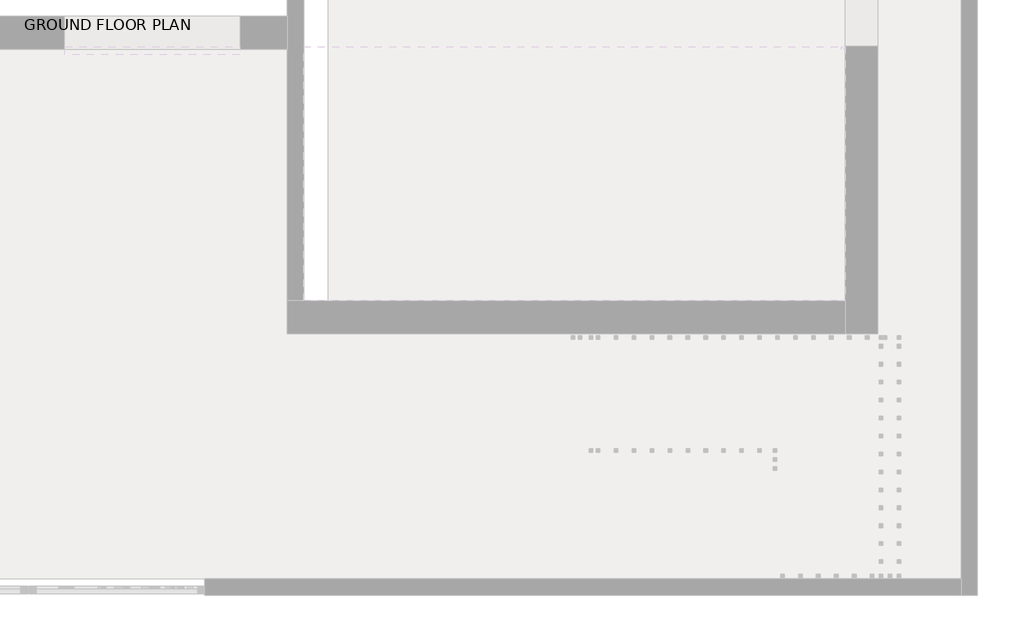
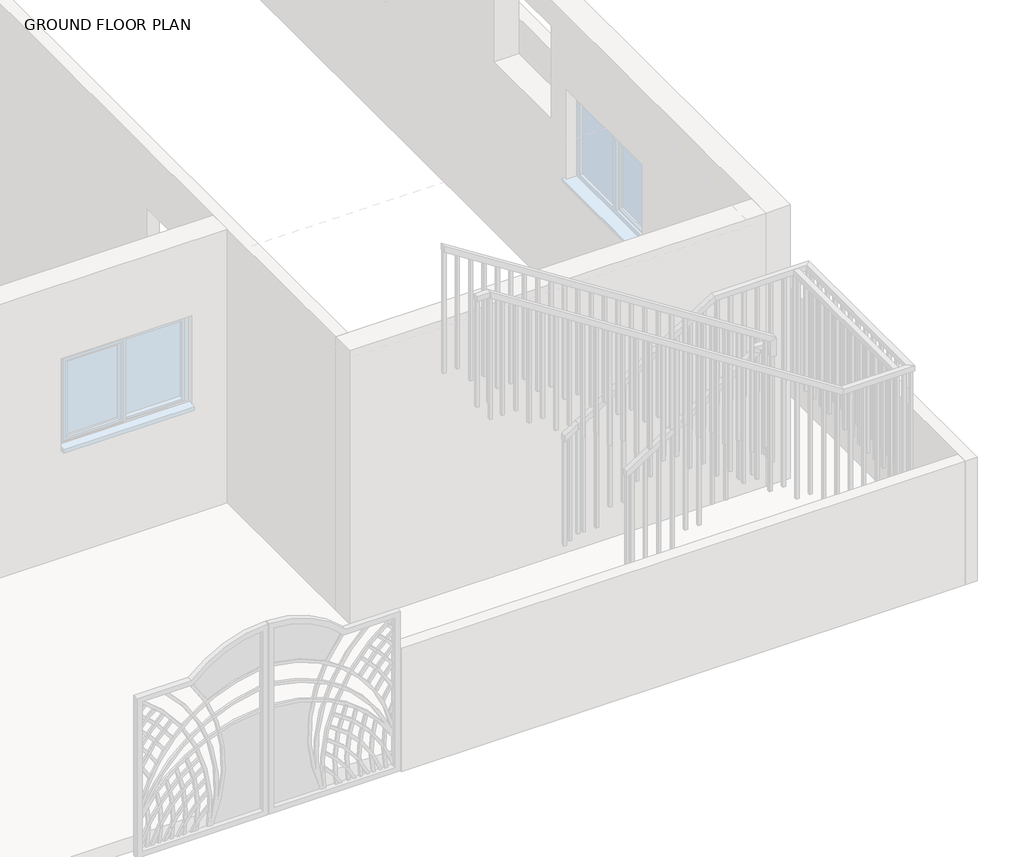
# One storey, part 4 of 23: 2 railings.
"""IFC4 building model written with IfcOpenShell, lengths in millimetres."""

from ifc_helpers import new_model, si_unit, frame, origin, place, context, project, spatial, polyline, outline, extrude, faceted_brep, element, save

model = new_model("IFC4")

# Units and contexts
model_context = context("Model", 3, world=origin())
ifc_project = project(units=[si_unit("LENGTHUNIT", "METRE", prefix="MILLI")], contexts=[model_context])

# Site, building, storey
site = spatial("IfcSite", under=ifc_project)
building = spatial("IfcBuilding", under=site)
storey = spatial("IfcBuildingStorey", under=building, Name="GROUND FLOOR PLAN", Elevation=487.68)

# Railings
placement = place(None, origin())
element("IfcRailing", 1, ObjectType="1100mm", at=placement, inside=storey, context=model_context, shape_type="SolidModel", body=[
    faceted_brep([(-8680.149573, -11007.9255223, 1912.8), (-8680.149573, -11007.9255223, 1853.4423995), (-8680.149573, -11057.9255223, 1853.4423995), (-8680.149573, -11057.9255223, 1912.8), (-7484.3306254, -11007.9255223, 2677.8717446), (-7434.3306254, -11007.9255223, 2650.5035914), (-7434.3306254, -11057.9255223, 2650.5035914), (-7484.3306254, -11057.9255223, 2677.8717446), (-7484.3306254, -11007.9255223, 2725.6), (-7434.3306254, -11007.9255223, 2675.6), (-7434.3306254, -11057.9255223, 2675.6), (-7484.3306254, -11057.9255223, 2725.6), (-7359.3306254, -11007.9255223, 2725.6), (-7359.3306254, -11007.9255223, 2675.6), (-7409.3306254, -11057.9255223, 2675.6), (-7409.3306254, -11057.9255223, 2725.6), (-7359.3306254, -11132.9255223, 2725.6), (-7359.3306254, -11132.9255223, 2675.6), (-7409.3306254, -11132.9255223, 2675.6), (-7409.3306254, -11132.9255223, 2725.6), (-7359.3306254, -11134.9255223, 2725.6), (-7409.3306254, -11134.9255223, 2725.6), (-7409.3306254, -11184.9255223, 2675.6), (-7359.3306254, -11184.9255223, 2675.6)], [[[0, 1, 2, 3]], [[1, 0, 4, 5]], [[2, 1, 5, 6]], [[3, 2, 6, 7]], [[0, 3, 7, 4]], [[5, 4, 8, 9]], [[6, 5, 9, 10]], [[7, 6, 10, 11]], [[4, 7, 11, 8]], [[9, 8, 12, 13]], [[10, 9, 13, 14]], [[11, 10, 14, 15]], [[8, 11, 15, 12]], [[13, 12, 16, 17]], [[14, 13, 17, 18]], [[15, 14, 18, 19]], [[12, 15, 19, 16]], [[20, 21, 22, 23]], [[17, 16, 20, 23]], [[18, 17, 23, 22]], [[19, 18, 22, 21]], [[16, 19, 21, 20]]]),
    faceted_brep([(-7359.3306254, -11134.9255223, 2725.6), (-7359.3306254, -11184.9255223, 2675.6), (-7409.3306254, -11184.9255223, 2675.6), (-7409.3306254, -11134.9255223, 2725.6), (-7359.3306254, -11134.9255223, 2855.9055527), (-7409.3306254, -11134.9255223, 2828.5415543), (-7409.3306254, -11184.9255223, 2828.5415543), (-7359.3306254, -11184.9255223, 2855.9055527)], [[[0, 1, 2, 3]], [[4, 5, 6, 7]], [[1, 0, 4, 7]], [[2, 1, 7, 6]], [[3, 2, 6, 5]], [[0, 3, 5, 4]]]),
    faceted_brep([(-7359.3306254, -11184.9255223, 2855.9055527), (-7409.3306254, -11184.9255223, 2828.5415543), (-7409.3306254, -11134.9255223, 2828.5415543), (-7359.3306254, -11134.9255223, 2855.9055527), (-10457.8773536, -11184.9255223, 4838.88), (-10457.8773536, -11134.9255223, 4838.88), (-10457.8773536, -11134.9255223, 4779.517542), (-10457.8773536, -11184.9255223, 4779.517542)], [[[0, 1, 2, 3]], [[4, 5, 6, 7]], [[1, 0, 4, 7]], [[2, 1, 7, 6]], [[3, 2, 6, 5]], [[0, 3, 5, 4]]]),
    extrude(outline(polyline([(3576.32, -10434.3306254), (4764.4483614, -10434.3306254), (4780.4475912, -10459.3306254), (3576.32, -10459.3306254), (3576.32, -10434.3306254)])), frame((0.0, -11172.4255223, 0.0), z_axis=(0.0, 1.0, 0.0), x_axis=(0.0, 0.0, 1.0)), (0.0, 0.0, 1.0), 25.0),
    extrude(outline(polyline([(3576.32, -10309.3306254), (4684.4522123, -10309.3306254), (4700.4514422, -10334.3306254), (3576.32, -10334.3306254), (3576.32, -10309.3306254)])), frame((0.0, -11172.4255223, 0.0), z_axis=(0.0, 1.0, 0.0), x_axis=(0.0, 0.0, 1.0)), (0.0, 0.0, 1.0), 25.0),
    extrude(outline(polyline([(3413.76, -10184.3306254), (4604.4560633, -10184.3306254), (4620.4552931, -10209.3306254), (3413.76, -10209.3306254), (3413.76, -10184.3306254)])), frame((0.0, -11172.4255223, 0.0), z_axis=(0.0, 1.0, 0.0), x_axis=(0.0, 0.0, 1.0)), (0.0, 0.0, 1.0), 25.0),
    extrude(outline(polyline([(3413.76, -10059.3306254), (4524.4599142, -10059.3306254), (4540.459144, -10084.3306254), (3413.76, -10084.3306254), (3413.76, -10059.3306254)])), frame((0.0, -11172.4255223, 0.0), z_axis=(0.0, 1.0, 0.0), x_axis=(0.0, 0.0, 1.0)), (0.0, 0.0, 1.0), 25.0),
    extrude(outline(polyline([(3251.2, -9934.3306254), (4444.4637652, -9934.3306254), (4460.462995, -9959.3306254), (3251.2, -9959.3306254), (3251.2, -9934.3306254)])), frame((0.0, -11172.4255223, 0.0), z_axis=(0.0, 1.0, 0.0), x_axis=(0.0, 0.0, 1.0)), (0.0, 0.0, 1.0), 25.0),
    extrude(outline(polyline([(3251.2, -9809.3306254), (4364.4676161, -9809.3306254), (4380.4668459, -9834.3306254), (3251.2, -9834.3306254), (3251.2, -9809.3306254)])), frame((0.0, -11172.4255223, 0.0), z_axis=(0.0, 1.0, 0.0), x_axis=(0.0, 0.0, 1.0)), (0.0, 0.0, 1.0), 25.0),
    extrude(outline(polyline([(3251.2, -9684.3306254), (4284.4714671, -9684.3306254), (4300.4706969, -9709.3306254), (3251.2, -9709.3306254), (3251.2, -9684.3306254)])), frame((0.0, -11172.4255223, 0.0), z_axis=(0.0, 1.0, 0.0), x_axis=(0.0, 0.0, 1.0)), (0.0, 0.0, 1.0), 25.0),
    extrude(outline(polyline([(3088.64, -9559.3306254), (4204.475318, -9559.3306254), (4220.4745478, -9584.3306254), (3088.64, -9584.3306254), (3088.64, -9559.3306254)])), frame((0.0, -11172.4255223, 0.0), z_axis=(0.0, 1.0, 0.0), x_axis=(0.0, 0.0, 1.0)), (0.0, 0.0, 1.0), 25.0),
    extrude(outline(polyline([(3088.64, -9434.3306254), (4124.479169, -9434.3306254), (4140.4783988, -9459.3306254), (3088.64, -9459.3306254), (3088.64, -9434.3306254)])), frame((0.0, -11172.4255223, 0.0), z_axis=(0.0, 1.0, 0.0), x_axis=(0.0, 0.0, 1.0)), (0.0, 0.0, 1.0), 25.0),
    extrude(outline(polyline([(2926.08, -9309.3306254), (4044.4830199, -9309.3306254), (4060.4822497, -9334.3306254), (2926.08, -9334.3306254), (2926.08, -9309.3306254)])), frame((0.0, -11172.4255223, 0.0), z_axis=(0.0, 1.0, 0.0), x_axis=(0.0, 0.0, 1.0)), (0.0, 0.0, 1.0), 25.0),
    extrude(outline(polyline([(2926.08, -9184.3306254), (3964.4868709, -9184.3306254), (3980.4861007, -9209.3306254), (2926.08, -9209.3306254), (2926.08, -9184.3306254)])), frame((0.0, -11172.4255223, 0.0), z_axis=(0.0, 1.0, 0.0), x_axis=(0.0, 0.0, 1.0)), (0.0, 0.0, 1.0), 25.0),
    extrude(outline(polyline([(2763.52, -9059.3306254), (3884.4907218, -9059.3306254), (3900.4899516, -9084.3306254), (2763.52, -9084.3306254), (2763.52, -9059.3306254)])), frame((0.0, -11172.4255223, 0.0), z_axis=(0.0, 1.0, 0.0), x_axis=(0.0, 0.0, 1.0)), (0.0, 0.0, 1.0), 25.0),
    extrude(outline(polyline([(2763.52, -8934.3306254), (3804.4945728, -8934.3306254), (3820.4938026, -8959.3306254), (2763.52, -8959.3306254), (2763.52, -8934.3306254)])), frame((0.0, -11172.4255223, 0.0), z_axis=(0.0, 1.0, 0.0), x_axis=(0.0, 0.0, 1.0)), (0.0, 0.0, 1.0), 25.0),
    extrude(outline(polyline([(2600.96, -8809.3306254), (3724.4984237, -8809.3306254), (3740.4976535, -8834.3306254), (2600.96, -8834.3306254), (2600.96, -8809.3306254)])), frame((0.0, -11172.4255223, 0.0), z_axis=(0.0, 1.0, 0.0), x_axis=(0.0, 0.0, 1.0)), (0.0, 0.0, 1.0), 25.0),
    extrude(outline(polyline([(2600.96, -8684.3306254), (3644.5022747, -8684.3306254), (3660.5015045, -8709.3306254), (2600.96, -8709.3306254), (2600.96, -8684.3306254)])), frame((0.0, -11172.4255223, 0.0), z_axis=(0.0, 1.0, 0.0), x_axis=(0.0, 0.0, 1.0)), (0.0, 0.0, 1.0), 25.0),
    extrude(outline(polyline([(2438.4, -8559.3306254), (3564.5061256, -8559.3306254), (3580.5053554, -8584.3306254), (2438.4, -8584.3306254), (2438.4, -8559.3306254)])), frame((0.0, -11172.4255223, 0.0), z_axis=(0.0, 1.0, 0.0), x_axis=(0.0, 0.0, 1.0)), (0.0, 0.0, 1.0), 25.0),
    extrude(outline(polyline([(2438.4, -8434.3306254), (3484.5099766, -8434.3306254), (3500.5092064, -8459.3306254), (2438.4, -8459.3306254), (2438.4, -8434.3306254)])), frame((0.0, -11172.4255223, 0.0), z_axis=(0.0, 1.0, 0.0), x_axis=(0.0, 0.0, 1.0)), (0.0, 0.0, 1.0), 25.0),
    extrude(outline(polyline([(2275.84, -8309.3306254), (3404.5138275, -8309.3306254), (3420.5130573, -8334.3306254), (2275.84, -8334.3306254), (2275.84, -8309.3306254)])), frame((0.0, -11172.4255223, 0.0), z_axis=(0.0, 1.0, 0.0), x_axis=(0.0, 0.0, 1.0)), (0.0, 0.0, 1.0), 25.0),
    extrude(outline(polyline([(2275.84, -8184.3306254), (3324.5176785, -8184.3306254), (3340.5169083, -8209.3306254), (2275.84, -8209.3306254), (2275.84, -8184.3306254)])), frame((0.0, -11172.4255223, 0.0), z_axis=(0.0, 1.0, 0.0), x_axis=(0.0, 0.0, 1.0)), (0.0, 0.0, 1.0), 25.0),
    extrude(outline(polyline([(2113.28, -8059.3306254), (3244.5215294, -8059.3306254), (3260.5207592, -8084.3306254), (2113.28, -8084.3306254), (2113.28, -8059.3306254)])), frame((0.0, -11172.4255223, 0.0), z_axis=(0.0, 1.0, 0.0), x_axis=(0.0, 0.0, 1.0)), (0.0, 0.0, 1.0), 25.0),
    extrude(outline(polyline([(2113.28, -7934.3306254), (3164.5253804, -7934.3306254), (3180.5246102, -7959.3306254), (2113.28, -7959.3306254), (2113.28, -7934.3306254)])), frame((0.0, -11172.4255223, 0.0), z_axis=(0.0, 1.0, 0.0), x_axis=(0.0, 0.0, 1.0)), (0.0, 0.0, 1.0), 25.0),
    extrude(outline(polyline([(1950.72, -7809.3306254), (3084.5292313, -7809.3306254), (3100.5284611, -7834.3306254), (1950.72, -7834.3306254), (1950.72, -7809.3306254)])), frame((0.0, -11172.4255223, 0.0), z_axis=(0.0, 1.0, 0.0), x_axis=(0.0, 0.0, 1.0)), (0.0, 0.0, 1.0), 25.0),
    extrude(outline(polyline([(1950.72, -7684.3306254), (3004.5330823, -7684.3306254), (3020.5323121, -7709.3306254), (1950.72, -7709.3306254), (1950.72, -7684.3306254)])), frame((0.0, -11172.4255223, 0.0), z_axis=(0.0, 1.0, 0.0), x_axis=(0.0, 0.0, 1.0)), (0.0, 0.0, 1.0), 25.0),
    extrude(outline(polyline([(1788.16, -7559.3306254), (2924.5369332, -7559.3306254), (2940.536163, -7584.3306254), (1788.16, -7584.3306254), (1788.16, -7559.3306254)])), frame((0.0, -11172.4255223, 0.0), z_axis=(0.0, 1.0, 0.0), x_axis=(0.0, 0.0, 1.0)), (0.0, 0.0, 1.0), 25.0),
    extrude(outline(polyline([(1788.16, -7434.3306254), (2844.5407841, -7434.3306254), (2860.540014, -7459.3306254), (1788.16, -7459.3306254), (1788.16, -7434.3306254)])), frame((0.0, -11172.4255223, 0.0), z_axis=(0.0, 1.0, 0.0), x_axis=(0.0, 0.0, 1.0)), (0.0, 0.0, 1.0), 25.0),
    extrude(outline(polyline([(-7396.8306254, -11082.9255223), (-7371.8306254, -11082.9255223), (-7371.8306254, -11107.9255223), (-7396.8306254, -11107.9255223), (-7396.8306254, -11082.9255223)])), frame((0.0, 0.0, 1625.6), z_axis=(0.0, 0.0, 1.0), x_axis=(1.0, 0.0, 0.0)), (0.0, 0.0, 1.0), 1050.0),
    extrude(outline(polyline([(2605.1944115, -7505.149573), (1463.04, -7505.149573), (1463.04, -7480.149573), (2621.1891352, -7480.149573), (2605.1944115, -7505.149573)])), frame((0.0, -11045.4255223, 0.0), z_axis=(0.0, 1.0, 0.0), x_axis=(0.0, 0.0, 1.0)), (0.0, 0.0, 1.0), 25.0),
    extrude(outline(polyline([(2525.2207932, -7630.149573), (1463.04, -7630.149573), (1463.04, -7605.149573), (2541.2155169, -7605.149573), (2525.2207932, -7630.149573)])), frame((0.0, -11045.4255223, 0.0), z_axis=(0.0, 1.0, 0.0), x_axis=(0.0, 0.0, 1.0)), (0.0, 0.0, 1.0), 25.0),
    extrude(outline(polyline([(2445.2471749, -7755.149573), (1300.48, -7755.149573), (1300.48, -7730.149573), (2461.2418986, -7730.149573), (2445.2471749, -7755.149573)])), frame((0.0, -11045.4255223, 0.0), z_axis=(0.0, 1.0, 0.0), x_axis=(0.0, 0.0, 1.0)), (0.0, 0.0, 1.0), 25.0),
    extrude(outline(polyline([(2365.2735566, -7880.149573), (1300.48, -7880.149573), (1300.48, -7855.149573), (2381.2682803, -7855.149573), (2365.2735566, -7880.149573)])), frame((0.0, -11045.4255223, 0.0), z_axis=(0.0, 1.0, 0.0), x_axis=(0.0, 0.0, 1.0)), (0.0, 0.0, 1.0), 25.0),
    extrude(outline(polyline([(2285.2999383, -8005.149573), (1137.92, -8005.149573), (1137.92, -7980.149573), (2301.294662, -7980.149573), (2285.2999383, -8005.149573)])), frame((0.0, -11045.4255223, 0.0), z_axis=(0.0, 1.0, 0.0), x_axis=(0.0, 0.0, 1.0)), (0.0, 0.0, 1.0), 25.0),
    extrude(outline(polyline([(2205.32632, -8130.149573), (1137.92, -8130.149573), (1137.92, -8105.149573), (2221.3210437, -8105.149573), (2205.32632, -8130.149573)])), frame((0.0, -11045.4255223, 0.0), z_axis=(0.0, 1.0, 0.0), x_axis=(0.0, 0.0, 1.0)), (0.0, 0.0, 1.0), 25.0),
    extrude(outline(polyline([(2125.3527017, -8255.149573), (975.36, -8255.149573), (975.36, -8230.149573), (2141.3474254, -8230.149573), (2125.3527017, -8255.149573)])), frame((0.0, -11045.4255223, 0.0), z_axis=(0.0, 1.0, 0.0), x_axis=(0.0, 0.0, 1.0)), (0.0, 0.0, 1.0), 25.0),
    extrude(outline(polyline([(2045.3790834, -8380.149573), (975.36, -8380.149573), (975.36, -8355.149573), (2061.3738071, -8355.149573), (2045.3790834, -8380.149573)])), frame((0.0, -11045.4255223, 0.0), z_axis=(0.0, 1.0, 0.0), x_axis=(0.0, 0.0, 1.0)), (0.0, 0.0, 1.0), 25.0),
    extrude(outline(polyline([(1965.4054651, -8505.149573), (812.8, -8505.149573), (812.8, -8480.149573), (1981.4001888, -8480.149573), (1965.4054651, -8505.149573)])), frame((0.0, -11045.4255223, 0.0), z_axis=(0.0, 1.0, 0.0), x_axis=(0.0, 0.0, 1.0)), (0.0, 0.0, 1.0), 25.0),
    extrude(outline(polyline([(1885.4318468, -8630.149573), (812.8, -8630.149573), (812.8, -8605.149573), (1901.4265705, -8605.149573), (1885.4318468, -8630.149573)])), frame((0.0, -11045.4255223, 0.0), z_axis=(0.0, 1.0, 0.0), x_axis=(0.0, 0.0, 1.0)), (0.0, 0.0, 1.0), 25.0),
    extrude(outline(polyline([(-7396.8306254, -11147.4255223), (-7371.8306254, -11147.4255223), (-7371.8306254, -11172.4255223), (-7396.8306254, -11172.4255223), (-7396.8306254, -11147.4255223)])), frame((0.0, 0.0, 1625.6), z_axis=(0.0, 0.0, 1.0), x_axis=(1.0, 0.0, 0.0)), (0.0, 0.0, 1.0), 1050.0),
    extrude(outline(polyline([(-7396.8306254, -11045.4255223), (-7396.8306254, -11020.4255223), (-7371.8306254, -11020.4255223), (-7371.8306254, -11045.4255223), (-7396.8306254, -11045.4255223)])), frame((0.0, 0.0, 1625.6), z_axis=(0.0, 0.0, 1.0), x_axis=(1.0, 0.0, 0.0)), (0.0, 0.0, 1.0), 1050.0),
    extrude(outline(polyline([(3576.32, -10432.8773536), (4763.5183122, -10432.8773536), (4779.517542, -10457.8773536), (3576.32, -10457.8773536), (3576.32, -10432.8773536)])), frame((0.0, -11172.4255223, 0.0), z_axis=(0.0, 1.0, 0.0), x_axis=(0.0, 0.0, 1.0)), (0.0, 0.0, 1.0), 25.0),
    extrude(outline(polyline([(1853.4423995, -8680.149573), (812.8, -8680.149573), (812.8, -8655.149573), (1869.4371231, -8655.149573), (1853.4423995, -8680.149573)])), frame((0.0, -11045.4255223, 0.0), z_axis=(0.0, 1.0, 0.0), x_axis=(0.0, 0.0, 1.0)), (0.0, 0.0, 1.0), 25.0),
])
element("IfcRailing", 2, ObjectType="1100mm", at=placement, inside=storey, context=model_context, shape_type="SolidModel", body=[
    faceted_brep([(-8680.149573, -10220.0521308, 1912.8), (-8680.149573, -10220.0521308, 1853.4423995), (-8680.149573, -10270.0521308, 1853.4423995), (-8680.149573, -10270.0521308, 1912.8), (-7409.7306254, -10220.0521308, 2725.6), (-7395.1045513, -10220.0521308, 2675.6), (-7395.1045513, -10270.0521308, 2675.6), (-7409.7306254, -10270.0521308, 2725.6), (-6495.8132565, -10220.0521308, 2725.6), (-6495.8132565, -10220.0521308, 2675.6), (-6545.8132565, -10270.0521308, 2675.6), (-6545.8132565, -10270.0521308, 2725.6), (-6495.8132565, -11933.6860066, 2725.6), (-6495.8132565, -11933.6860066, 2675.6), (-6545.8132565, -11883.6860066, 2675.6), (-6545.8132565, -11883.6860066, 2725.6), (-7155.718398, -11933.6860066, 2725.6), (-7170.3479429, -11933.6860066, 2675.6), (-7170.3479429, -11883.6860066, 2675.6), (-7155.718398, -11883.6860066, 2725.6), (-10457.8773536, -11933.6860066, 4838.88), (-10457.8773536, -11883.6860066, 4838.88), (-10457.8773536, -11883.6860066, 4779.517542), (-10457.8773536, -11933.6860066, 4779.517542)], [[[0, 1, 2, 3]], [[1, 0, 4, 5]], [[2, 1, 5, 6]], [[3, 2, 6, 7]], [[0, 3, 7, 4]], [[5, 4, 8, 9]], [[6, 5, 9, 10]], [[7, 6, 10, 11]], [[4, 7, 11, 8]], [[9, 8, 12, 13]], [[10, 9, 13, 14]], [[11, 10, 14, 15]], [[8, 11, 15, 12]], [[13, 12, 16, 17]], [[14, 13, 17, 18]], [[15, 14, 18, 19]], [[12, 15, 19, 16]], [[20, 21, 22, 23]], [[17, 16, 20, 23]], [[18, 17, 23, 22]], [[19, 18, 22, 21]], [[16, 19, 21, 20]]]),
    extrude(outline(polyline([(4691.8007425, -10320.8132565), (4707.7999723, -10345.8132565), (3576.32, -10345.8132565), (3576.32, -10320.8132565), (4691.8007425, -10320.8132565)])), frame((0.0, -11921.1860066, 0.0), z_axis=(0.0, 1.0, 0.0), x_axis=(0.0, 0.0, 1.0)), (0.0, 0.0, 1.0), 25.0),
    extrude(outline(polyline([(4611.8045935, -10195.8132565), (4627.8038233, -10220.8132565), (3576.32, -10220.8132565), (3576.32, -10195.8132565), (4611.8045935, -10195.8132565)])), frame((0.0, -11921.1860066, 0.0), z_axis=(0.0, 1.0, 0.0), x_axis=(0.0, 0.0, 1.0)), (0.0, 0.0, 1.0), 25.0),
    extrude(outline(polyline([(4531.8084444, -10070.8132565), (4547.8076742, -10095.8132565), (3413.76, -10095.8132565), (3413.76, -10070.8132565), (4531.8084444, -10070.8132565)])), frame((0.0, -11921.1860066, 0.0), z_axis=(0.0, 1.0, 0.0), x_axis=(0.0, 0.0, 1.0)), (0.0, 0.0, 1.0), 25.0),
    extrude(outline(polyline([(4451.8122954, -9945.8132565), (4467.8115252, -9970.8132565), (3413.76, -9970.8132565), (3413.76, -9945.8132565), (4451.8122954, -9945.8132565)])), frame((0.0, -11921.1860066, 0.0), z_axis=(0.0, 1.0, 0.0), x_axis=(0.0, 0.0, 1.0)), (0.0, 0.0, 1.0), 25.0),
    extrude(outline(polyline([(4371.8161463, -9820.8132565), (4387.8153761, -9845.8132565), (3251.2, -9845.8132565), (3251.2, -9820.8132565), (4371.8161463, -9820.8132565)])), frame((0.0, -11921.1860066, 0.0), z_axis=(0.0, 1.0, 0.0), x_axis=(0.0, 0.0, 1.0)), (0.0, 0.0, 1.0), 25.0),
    extrude(outline(polyline([(4291.8423995, -9695.8132565), (4307.8371231, -9720.8132565), (3251.2, -9720.8132565), (3251.2, -9695.8132565), (4291.8423995, -9695.8132565)])), frame((0.0, -11921.1860066, 0.0), z_axis=(0.0, 1.0, 0.0), x_axis=(0.0, 0.0, 1.0)), (0.0, 0.0, 1.0), 25.0),
    extrude(outline(polyline([(4211.8238482, -9570.8132565), (4227.823078, -9595.8132565), (3088.64, -9595.8132565), (3088.64, -9570.8132565), (4211.8238482, -9570.8132565)])), frame((0.0, -11921.1860066, 0.0), z_axis=(0.0, 1.0, 0.0), x_axis=(0.0, 0.0, 1.0)), (0.0, 0.0, 1.0), 25.0),
    extrude(outline(polyline([(4131.8276992, -9445.8132565), (4147.826929, -9470.8132565), (3088.64, -9470.8132565), (3088.64, -9445.8132565), (4131.8276992, -9445.8132565)])), frame((0.0, -11921.1860066, 0.0), z_axis=(0.0, 1.0, 0.0), x_axis=(0.0, 0.0, 1.0)), (0.0, 0.0, 1.0), 25.0),
    extrude(outline(polyline([(4051.8315501, -9320.8132565), (4067.8307799, -9345.8132565), (2926.08, -9345.8132565), (2926.08, -9320.8132565), (4051.8315501, -9320.8132565)])), frame((0.0, -11921.1860066, 0.0), z_axis=(0.0, 1.0, 0.0), x_axis=(0.0, 0.0, 1.0)), (0.0, 0.0, 1.0), 25.0),
    extrude(outline(polyline([(3971.835401, -9195.8132565), (3987.8346309, -9220.8132565), (2926.08, -9220.8132565), (2926.08, -9195.8132565), (3971.835401, -9195.8132565)])), frame((0.0, -11921.1860066, 0.0), z_axis=(0.0, 1.0, 0.0), x_axis=(0.0, 0.0, 1.0)), (0.0, 0.0, 1.0), 25.0),
    extrude(outline(polyline([(3891.839252, -9070.8132565), (3907.8384818, -9095.8132565), (2763.52, -9095.8132565), (2763.52, -9070.8132565), (3891.839252, -9070.8132565)])), frame((0.0, -11921.1860066, 0.0), z_axis=(0.0, 1.0, 0.0), x_axis=(0.0, 0.0, 1.0)), (0.0, 0.0, 1.0), 25.0),
    extrude(outline(polyline([(3811.8431029, -8945.8132565), (3827.8423328, -8970.8132565), (2763.52, -8970.8132565), (2763.52, -8945.8132565), (3811.8431029, -8945.8132565)])), frame((0.0, -11921.1860066, 0.0), z_axis=(0.0, 1.0, 0.0), x_axis=(0.0, 0.0, 1.0)), (0.0, 0.0, 1.0), 25.0),
    extrude(outline(polyline([(3731.8469539, -8820.8132565), (3747.8461837, -8845.8132565), (2600.96, -8845.8132565), (2600.96, -8820.8132565), (3731.8469539, -8820.8132565)])), frame((0.0, -11921.1860066, 0.0), z_axis=(0.0, 1.0, 0.0), x_axis=(0.0, 0.0, 1.0)), (0.0, 0.0, 1.0), 25.0),
    extrude(outline(polyline([(3651.8508048, -8695.8132565), (3667.8500347, -8720.8132565), (2600.96, -8720.8132565), (2600.96, -8695.8132565), (3651.8508048, -8695.8132565)])), frame((0.0, -11921.1860066, 0.0), z_axis=(0.0, 1.0, 0.0), x_axis=(0.0, 0.0, 1.0)), (0.0, 0.0, 1.0), 25.0),
    extrude(outline(polyline([(3571.8546558, -8570.8132565), (3587.8538856, -8595.8132565), (2438.4, -8595.8132565), (2438.4, -8570.8132565), (3571.8546558, -8570.8132565)])), frame((0.0, -11921.1860066, 0.0), z_axis=(0.0, 1.0, 0.0), x_axis=(0.0, 0.0, 1.0)), (0.0, 0.0, 1.0), 25.0),
    extrude(outline(polyline([(3491.8585067, -8445.8132565), (3507.8577365, -8470.8132565), (2438.4, -8470.8132565), (2438.4, -8445.8132565), (3491.8585067, -8445.8132565)])), frame((0.0, -11921.1860066, 0.0), z_axis=(0.0, 1.0, 0.0), x_axis=(0.0, 0.0, 1.0)), (0.0, 0.0, 1.0), 25.0),
    extrude(outline(polyline([(3411.8623577, -8320.8132565), (3427.8615875, -8345.8132565), (2275.84, -8345.8132565), (2275.84, -8320.8132565), (3411.8623577, -8320.8132565)])), frame((0.0, -11921.1860066, 0.0), z_axis=(0.0, 1.0, 0.0), x_axis=(0.0, 0.0, 1.0)), (0.0, 0.0, 1.0), 25.0),
    extrude(outline(polyline([(3331.8662086, -8195.8132565), (3347.8654384, -8220.8132565), (2275.84, -8220.8132565), (2275.84, -8195.8132565), (3331.8662086, -8195.8132565)])), frame((0.0, -11921.1860066, 0.0), z_axis=(0.0, 1.0, 0.0), x_axis=(0.0, 0.0, 1.0)), (0.0, 0.0, 1.0), 25.0),
    extrude(outline(polyline([(3251.8700596, -8070.8132565), (3267.8692894, -8095.8132565), (2113.28, -8095.8132565), (2113.28, -8070.8132565), (3251.8700596, -8070.8132565)])), frame((0.0, -11921.1860066, 0.0), z_axis=(0.0, 1.0, 0.0), x_axis=(0.0, 0.0, 1.0)), (0.0, 0.0, 1.0), 25.0),
    extrude(outline(polyline([(3171.8739105, -7945.8132565), (3187.8731403, -7970.8132565), (2113.28, -7970.8132565), (2113.28, -7945.8132565), (3171.8739105, -7945.8132565)])), frame((0.0, -11921.1860066, 0.0), z_axis=(0.0, 1.0, 0.0), x_axis=(0.0, 0.0, 1.0)), (0.0, 0.0, 1.0), 25.0),
    extrude(outline(polyline([(3091.8777615, -7820.8132565), (3107.8769913, -7845.8132565), (1950.72, -7845.8132565), (1950.72, -7820.8132565), (3091.8777615, -7820.8132565)])), frame((0.0, -11921.1860066, 0.0), z_axis=(0.0, 1.0, 0.0), x_axis=(0.0, 0.0, 1.0)), (0.0, 0.0, 1.0), 25.0),
    extrude(outline(polyline([(3011.8816124, -7695.8132565), (3027.8808422, -7720.8132565), (1950.72, -7720.8132565), (1950.72, -7695.8132565), (3011.8816124, -7695.8132565)])), frame((0.0, -11921.1860066, 0.0), z_axis=(0.0, 1.0, 0.0), x_axis=(0.0, 0.0, 1.0)), (0.0, 0.0, 1.0), 25.0),
    extrude(outline(polyline([(2931.8854634, -7570.8132565), (2947.8846932, -7595.8132565), (1788.16, -7595.8132565), (1788.16, -7570.8132565), (2931.8854634, -7570.8132565)])), frame((0.0, -11921.1860066, 0.0), z_axis=(0.0, 1.0, 0.0), x_axis=(0.0, 0.0, 1.0)), (0.0, 0.0, 1.0), 25.0),
    extrude(outline(polyline([(2851.8893143, -7445.8132565), (2867.8885441, -7470.8132565), (1788.16, -7470.8132565), (1788.16, -7445.8132565), (2851.8893143, -7445.8132565)])), frame((0.0, -11921.1860066, 0.0), z_axis=(0.0, 1.0, 0.0), x_axis=(0.0, 0.0, 1.0)), (0.0, 0.0, 1.0), 25.0),
    extrude(outline(polyline([(2771.8931653, -7320.8132565), (2787.8923951, -7345.8132565), (1625.6, -7345.8132565), (1625.6, -7320.8132565), (2771.8931653, -7320.8132565)])), frame((0.0, -11921.1860066, 0.0), z_axis=(0.0, 1.0, 0.0), x_axis=(0.0, 0.0, 1.0)), (0.0, 0.0, 1.0), 25.0),
    extrude(outline(polyline([(2691.8970162, -7195.8132565), (2707.896246, -7220.8132565), (1625.6, -7220.8132565), (1625.6, -7195.8132565), (2691.8970162, -7195.8132565)])), frame((0.0, -11921.1860066, 0.0), z_axis=(0.0, 1.0, 0.0), x_axis=(0.0, 0.0, 1.0)), (0.0, 0.0, 1.0), 25.0),
    extrude(outline(polyline([(-7070.8132565, -11921.1860066), (-7095.8132565, -11921.1860066), (-7095.8132565, -11896.1860066), (-7070.8132565, -11896.1860066), (-7070.8132565, -11921.1860066)])), frame((0.0, 0.0, 1625.6), z_axis=(0.0, 0.0, 1.0), x_axis=(1.0, 0.0, 0.0)), (0.0, 0.0, 1.0), 1050.0),
    extrude(outline(polyline([(-6945.8132565, -11921.1860066), (-6970.8132565, -11921.1860066), (-6970.8132565, -11896.1860066), (-6945.8132565, -11896.1860066), (-6945.8132565, -11921.1860066)])), frame((0.0, 0.0, 1625.6), z_axis=(0.0, 0.0, 1.0), x_axis=(1.0, 0.0, 0.0)), (0.0, 0.0, 1.0), 1050.0),
    extrude(outline(polyline([(-6820.8132565, -11921.1860066), (-6845.8132565, -11921.1860066), (-6845.8132565, -11896.1860066), (-6820.8132565, -11896.1860066), (-6820.8132565, -11921.1860066)])), frame((0.0, 0.0, 1625.6), z_axis=(0.0, 0.0, 1.0), x_axis=(1.0, 0.0, 0.0)), (0.0, 0.0, 1.0), 1050.0),
    extrude(outline(polyline([(-6695.8132565, -11921.1860066), (-6720.8132565, -11921.1860066), (-6720.8132565, -11896.1860066), (-6695.8132565, -11896.1860066), (-6695.8132565, -11921.1860066)])), frame((0.0, 0.0, 1625.6), z_axis=(0.0, 0.0, 1.0), x_axis=(1.0, 0.0, 0.0)), (0.0, 0.0, 1.0), 1050.0),
    extrude(outline(polyline([(-6570.8132565, -11921.1860066), (-6595.8132565, -11921.1860066), (-6595.8132565, -11896.1860066), (-6570.8132565, -11896.1860066), (-6570.8132565, -11921.1860066)])), frame((0.0, 0.0, 1625.6), z_axis=(0.0, 0.0, 1.0), x_axis=(1.0, 0.0, 0.0)), (0.0, 0.0, 1.0), 1050.0),
    extrude(outline(polyline([(-6508.3132565, -11795.0521308), (-6508.3132565, -11820.0521308), (-6533.3132565, -11820.0521308), (-6533.3132565, -11795.0521308), (-6508.3132565, -11795.0521308)])), frame((0.0, 0.0, 1625.6), z_axis=(0.0, 0.0, 1.0), x_axis=(1.0, 0.0, 0.0)), (0.0, 0.0, 1.0), 1050.0),
    extrude(outline(polyline([(-6508.3132565, -11670.0521308), (-6508.3132565, -11695.0521308), (-6533.3132565, -11695.0521308), (-6533.3132565, -11670.0521308), (-6508.3132565, -11670.0521308)])), frame((0.0, 0.0, 1625.6), z_axis=(0.0, 0.0, 1.0), x_axis=(1.0, 0.0, 0.0)), (0.0, 0.0, 1.0), 1050.0),
    extrude(outline(polyline([(-6508.3132565, -11545.0521308), (-6508.3132565, -11570.0521308), (-6533.3132565, -11570.0521308), (-6533.3132565, -11545.0521308), (-6508.3132565, -11545.0521308)])), frame((0.0, 0.0, 1625.6), z_axis=(0.0, 0.0, 1.0), x_axis=(1.0, 0.0, 0.0)), (0.0, 0.0, 1.0), 1050.0),
    extrude(outline(polyline([(-6508.3132565, -11420.0521308), (-6508.3132565, -11445.0521308), (-6533.3132565, -11445.0521308), (-6533.3132565, -11420.0521308), (-6508.3132565, -11420.0521308)])), frame((0.0, 0.0, 1625.6), z_axis=(0.0, 0.0, 1.0), x_axis=(1.0, 0.0, 0.0)), (0.0, 0.0, 1.0), 1050.0),
    extrude(outline(polyline([(-6508.3132565, -11295.0521308), (-6508.3132565, -11320.0521308), (-6533.3132565, -11320.0521308), (-6533.3132565, -11295.0521308), (-6508.3132565, -11295.0521308)])), frame((0.0, 0.0, 1625.6), z_axis=(0.0, 0.0, 1.0), x_axis=(1.0, 0.0, 0.0)), (0.0, 0.0, 1.0), 1050.0),
    extrude(outline(polyline([(-6508.3132565, -11170.0521308), (-6508.3132565, -11195.0521308), (-6533.3132565, -11195.0521308), (-6533.3132565, -11170.0521308), (-6508.3132565, -11170.0521308)])), frame((0.0, 0.0, 1625.6), z_axis=(0.0, 0.0, 1.0), x_axis=(1.0, 0.0, 0.0)), (0.0, 0.0, 1.0), 1050.0),
    extrude(outline(polyline([(-6508.3132565, -11045.0521308), (-6508.3132565, -11070.0521308), (-6533.3132565, -11070.0521308), (-6533.3132565, -11045.0521308), (-6508.3132565, -11045.0521308)])), frame((0.0, 0.0, 1625.6), z_axis=(0.0, 0.0, 1.0), x_axis=(1.0, 0.0, 0.0)), (0.0, 0.0, 1.0), 1050.0),
    extrude(outline(polyline([(-6508.3132565, -10920.0521308), (-6508.3132565, -10945.0521308), (-6533.3132565, -10945.0521308), (-6533.3132565, -10920.0521308), (-6508.3132565, -10920.0521308)])), frame((0.0, 0.0, 1625.6), z_axis=(0.0, 0.0, 1.0), x_axis=(1.0, 0.0, 0.0)), (0.0, 0.0, 1.0), 1050.0),
    extrude(outline(polyline([(-6508.3132565, -10795.0521308), (-6508.3132565, -10820.0521308), (-6533.3132565, -10820.0521308), (-6533.3132565, -10795.0521308), (-6508.3132565, -10795.0521308)])), frame((0.0, 0.0, 1625.6), z_axis=(0.0, 0.0, 1.0), x_axis=(1.0, 0.0, 0.0)), (0.0, 0.0, 1.0), 1050.0),
    extrude(outline(polyline([(-6508.3132565, -10670.0521308), (-6508.3132565, -10695.0521308), (-6533.3132565, -10695.0521308), (-6533.3132565, -10670.0521308), (-6508.3132565, -10670.0521308)])), frame((0.0, 0.0, 1625.6), z_axis=(0.0, 0.0, 1.0), x_axis=(1.0, 0.0, 0.0)), (0.0, 0.0, 1.0), 1050.0),
    extrude(outline(polyline([(-6508.3132565, -10545.0521308), (-6508.3132565, -10570.0521308), (-6533.3132565, -10570.0521308), (-6533.3132565, -10545.0521308), (-6508.3132565, -10545.0521308)])), frame((0.0, 0.0, 1625.6), z_axis=(0.0, 0.0, 1.0), x_axis=(1.0, 0.0, 0.0)), (0.0, 0.0, 1.0), 1050.0),
    extrude(outline(polyline([(-6508.3132565, -10420.0521308), (-6508.3132565, -10445.0521308), (-6533.3132565, -10445.0521308), (-6533.3132565, -10420.0521308), (-6508.3132565, -10420.0521308)])), frame((0.0, 0.0, 1625.6), z_axis=(0.0, 0.0, 1.0), x_axis=(1.0, 0.0, 0.0)), (0.0, 0.0, 1.0), 1050.0),
    extrude(outline(polyline([(-6508.3132565, -10295.0521308), (-6508.3132565, -10320.0521308), (-6533.3132565, -10320.0521308), (-6533.3132565, -10295.0521308), (-6508.3132565, -10295.0521308)])), frame((0.0, 0.0, 1625.6), z_axis=(0.0, 0.0, 1.0), x_axis=(1.0, 0.0, 0.0)), (0.0, 0.0, 1.0), 1050.0),
    extrude(outline(polyline([(-6630.149573, -10232.5521308), (-6605.149573, -10232.5521308), (-6605.149573, -10257.5521308), (-6630.149573, -10257.5521308), (-6630.149573, -10232.5521308)])), frame((0.0, 0.0, 1625.6), z_axis=(0.0, 0.0, 1.0), x_axis=(1.0, 0.0, 0.0)), (0.0, 0.0, 1.0), 1050.0),
    extrude(outline(polyline([(-6755.149573, -10232.5521308), (-6730.149573, -10232.5521308), (-6730.149573, -10257.5521308), (-6755.149573, -10257.5521308), (-6755.149573, -10232.5521308)])), frame((0.0, 0.0, 1625.6), z_axis=(0.0, 0.0, 1.0), x_axis=(1.0, 0.0, 0.0)), (0.0, 0.0, 1.0), 1050.0),
    extrude(outline(polyline([(-6880.149573, -10232.5521308), (-6855.149573, -10232.5521308), (-6855.149573, -10257.5521308), (-6880.149573, -10257.5521308), (-6880.149573, -10232.5521308)])), frame((0.0, 0.0, 1625.6), z_axis=(0.0, 0.0, 1.0), x_axis=(1.0, 0.0, 0.0)), (0.0, 0.0, 1.0), 1050.0),
    extrude(outline(polyline([(-7005.149573, -10232.5521308), (-6980.149573, -10232.5521308), (-6980.149573, -10257.5521308), (-7005.149573, -10257.5521308), (-7005.149573, -10232.5521308)])), frame((0.0, 0.0, 1625.6), z_axis=(0.0, 0.0, 1.0), x_axis=(1.0, 0.0, 0.0)), (0.0, 0.0, 1.0), 1050.0),
    extrude(outline(polyline([(-7130.149573, -10232.5521308), (-7105.149573, -10232.5521308), (-7105.149573, -10257.5521308), (-7130.149573, -10257.5521308), (-7130.149573, -10232.5521308)])), frame((0.0, 0.0, 1625.6), z_axis=(0.0, 0.0, 1.0), x_axis=(1.0, 0.0, 0.0)), (0.0, 0.0, 1.0), 1050.0),
    extrude(outline(polyline([(-7255.149573, -10232.5521308), (-7230.149573, -10232.5521308), (-7230.149573, -10257.5521308), (-7255.149573, -10257.5521308), (-7255.149573, -10232.5521308)])), frame((0.0, 0.0, 1625.6), z_axis=(0.0, 0.0, 1.0), x_axis=(1.0, 0.0, 0.0)), (0.0, 0.0, 1.0), 1050.0),
    extrude(outline(polyline([(-7380.149573, -10232.5521308), (-7355.149573, -10232.5521308), (-7355.149573, -10257.5521308), (-7380.149573, -10257.5521308), (-7380.149573, -10232.5521308)])), frame((0.0, 0.0, 1625.6), z_axis=(0.0, 0.0, 1.0), x_axis=(1.0, 0.0, 0.0)), (0.0, 0.0, 1.0), 1050.0),
    extrude(outline(polyline([(1463.04, -7505.149573), (1463.04, -7480.149573), (2621.1891352, -7480.149573), (2605.1944115, -7505.149573), (1463.04, -7505.149573)])), frame((0.0, -10257.5521308, 0.0), z_axis=(0.0, 1.0, 0.0), x_axis=(0.0, 0.0, 1.0)), (0.0, 0.0, 1.0), 25.0),
    extrude(outline(polyline([(1463.04, -7630.149573), (1463.04, -7605.149573), (2541.2155169, -7605.149573), (2525.2207932, -7630.149573), (1463.04, -7630.149573)])), frame((0.0, -10257.5521308, 0.0), z_axis=(0.0, 1.0, 0.0), x_axis=(0.0, 0.0, 1.0)), (0.0, 0.0, 1.0), 25.0),
    extrude(outline(polyline([(1300.48, -7755.149573), (1300.48, -7730.149573), (2461.2418986, -7730.149573), (2445.2471749, -7755.149573), (1300.48, -7755.149573)])), frame((0.0, -10257.5521308, 0.0), z_axis=(0.0, 1.0, 0.0), x_axis=(0.0, 0.0, 1.0)), (0.0, 0.0, 1.0), 25.0),
    extrude(outline(polyline([(1300.48, -7880.149573), (1300.48, -7855.149573), (2381.2682803, -7855.149573), (2365.2735566, -7880.149573), (1300.48, -7880.149573)])), frame((0.0, -10257.5521308, 0.0), z_axis=(0.0, 1.0, 0.0), x_axis=(0.0, 0.0, 1.0)), (0.0, 0.0, 1.0), 25.0),
    extrude(outline(polyline([(1137.92, -8005.149573), (1137.92, -7980.149573), (2301.294662, -7980.149573), (2285.2999383, -8005.149573), (1137.92, -8005.149573)])), frame((0.0, -10257.5521308, 0.0), z_axis=(0.0, 1.0, 0.0), x_axis=(0.0, 0.0, 1.0)), (0.0, 0.0, 1.0), 25.0),
    extrude(outline(polyline([(1137.92, -8130.149573), (1137.92, -8105.149573), (2221.3210437, -8105.149573), (2205.32632, -8130.149573), (1137.92, -8130.149573)])), frame((0.0, -10257.5521308, 0.0), z_axis=(0.0, 1.0, 0.0), x_axis=(0.0, 0.0, 1.0)), (0.0, 0.0, 1.0), 25.0),
    extrude(outline(polyline([(975.36, -8255.149573), (975.36, -8230.149573), (2141.3474254, -8230.149573), (2125.3527017, -8255.149573), (975.36, -8255.149573)])), frame((0.0, -10257.5521308, 0.0), z_axis=(0.0, 1.0, 0.0), x_axis=(0.0, 0.0, 1.0)), (0.0, 0.0, 1.0), 25.0),
    extrude(outline(polyline([(975.36, -8380.149573), (975.36, -8355.149573), (2061.3738071, -8355.149573), (2045.3790834, -8380.149573), (975.36, -8380.149573)])), frame((0.0, -10257.5521308, 0.0), z_axis=(0.0, 1.0, 0.0), x_axis=(0.0, 0.0, 1.0)), (0.0, 0.0, 1.0), 25.0),
    extrude(outline(polyline([(812.8, -8505.149573), (812.8, -8480.149573), (1981.4001888, -8480.149573), (1965.4054651, -8505.149573), (812.8, -8505.149573)])), frame((0.0, -10257.5521308, 0.0), z_axis=(0.0, 1.0, 0.0), x_axis=(0.0, 0.0, 1.0)), (0.0, 0.0, 1.0), 25.0),
    extrude(outline(polyline([(812.8, -8630.149573), (812.8, -8605.149573), (1901.4265705, -8605.149573), (1885.4318468, -8630.149573), (812.8, -8630.149573)])), frame((0.0, -10257.5521308, 0.0), z_axis=(0.0, 1.0, 0.0), x_axis=(0.0, 0.0, 1.0)), (0.0, 0.0, 1.0), 25.0),
    extrude(outline(polyline([(-6508.3132565, -11896.1860066), (-6508.3132565, -11921.1860066), (-6533.3132565, -11921.1860066), (-6533.3132565, -11896.1860066), (-6508.3132565, -11896.1860066)])), frame((0.0, 0.0, 1625.6), z_axis=(0.0, 0.0, 1.0), x_axis=(1.0, 0.0, 0.0)), (0.0, 0.0, 1.0), 1050.0),
    extrude(outline(polyline([(-6533.3132565, -10232.5521308), (-6508.3132565, -10232.5521308), (-6508.3132565, -10257.5521308), (-6533.3132565, -10257.5521308), (-6533.3132565, -10232.5521308)])), frame((0.0, 0.0, 1625.6), z_axis=(0.0, 0.0, 1.0), x_axis=(1.0, 0.0, 0.0)), (0.0, 0.0, 1.0), 1050.0),
    extrude(outline(polyline([(4763.5183122, -10432.8773536), (4779.517542, -10457.8773536), (3576.32, -10457.8773536), (3576.32, -10432.8773536), (4763.5183122, -10432.8773536)])), frame((0.0, -11921.1860066, 0.0), z_axis=(0.0, 1.0, 0.0), x_axis=(0.0, 0.0, 1.0)), (0.0, 0.0, 1.0), 25.0),
    extrude(outline(polyline([(812.8, -8680.149573), (812.8, -8655.149573), (1869.4371231, -8655.149573), (1853.4423995, -8680.149573), (812.8, -8680.149573)])), frame((0.0, -10257.5521308, 0.0), z_axis=(0.0, 1.0, 0.0), x_axis=(0.0, 0.0, 1.0)), (0.0, 0.0, 1.0), 25.0),
])

save(model, "model.ifc")

# Revit data of these elements
# Type "1100mm"
#   built-in parameter 1008612 = 0.019685 (stored number, unit not read)
#   built-in parameter 1008611 = 0.019685 (stored number, unit not read)
#   built-in parameter 1008609 = 0.902231 (stored number, unit not read)
#   built-in parameter 1008604 = 0.19685 (stored number, unit not read)
#   built-in parameter 1008603 = 0.164042 (stored number, unit not read)
#   Railing Height = 3.608924 ft
#   built-in parameter 1008630 = 2
#   built-in parameter 1008610 = 2
#   built-in parameter 1008608 = 1
#   built-in parameter 1008618 = Baluster_Square : 25mm
# Elements 1, 2 (IfcRailing, "1100mm")
#   Phase Created = New Construction
